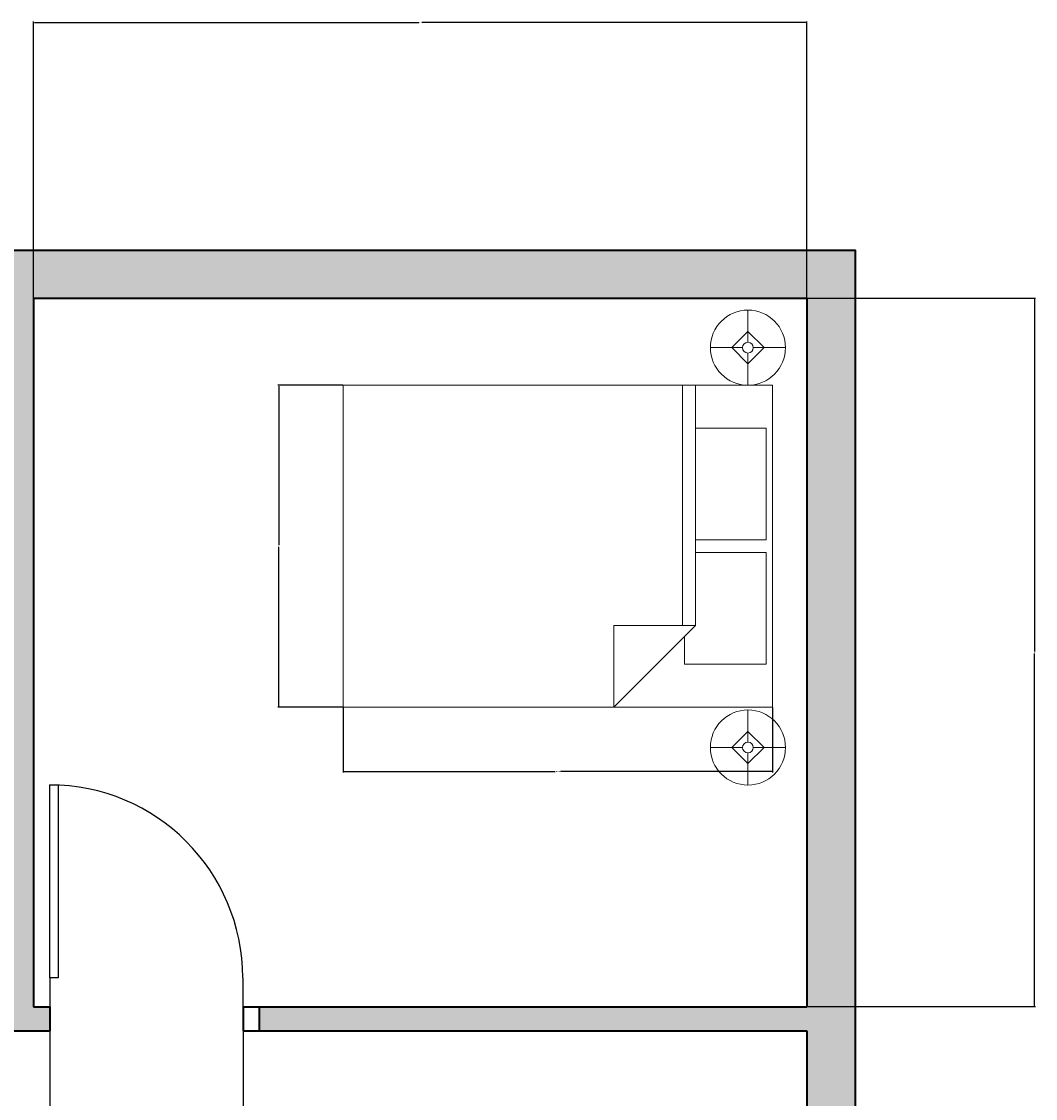
# Model space of a CAD drawing. Units: inches. Extents: x 1563 to 2428, y 777 to 1464.
# Tile 8 of 11: x 1810 to 1999, y 1263 to 1464. Entities that reach past the tile are written whole.
import ezdxf

# ---------------------------------------------------------------- set-up
doc = ezdxf.new("R2010")
doc.units = ezdxf.units.IN
for name, color, linetype, lineweight in [('A-ANNO-DIMS', 2, 'Continuous', 18), ('A-DOOR', 4, 'Continuous', 25), ('A-FURN', 9, 'Continuous', 18), ('A-WALL', 7, 'Continuous', 35), ('A-WALL-PATT', 8, 'Continuous', 13)]:
    doc.layers.add(name, color=color, linetype=linetype, lineweight=lineweight)
doc.styles.get("Standard").update_dxf_attribs({"font": 'arial.ttf'})
doc.dimstyles.get("Standard").update_dxf_attribs({"dimtxt": 0.18, "dimasz": 0.18, "dimexe": 0.18, "dimexo": 0.0625, "dimgap": 0.09, "dimtad": 0, "dimtih": 1, "dimtoh": 1, "dimdec": 4, "dimzin": 0, "dimdsep": 46, "dimtxsty": 'Standard', "dimcen": 0.09, "dimadec": 0, "dimazin": 0, "dimtfac": 1, "dimtdec": 4, "dimtofl": 0, "dimtmove": 0, "dimatfit": 3, "dimfxl": 1, "dimtolj": 1, "dimtzin": 0, "dimarcsym": 0})

# ---------------------------------------------------------------- blocks, each defined once
blk = doc.blocks.new('*U4')
for p, q in [((0, 0), (0, -6)), ((40, 0), (40, -6))]:
    blk.add_line(p, q)
blk.add_lwpolyline([(0, 0), (0, 40), (1.75, 40), (1.75, 0)], close=True)
blk.add_arc((0, 0), 40, 0, 90)
blk = doc.blocks.new('Bed - Queen')
for p, q in [((0, -80.00003), (0, 0)), ((0, 0), (59.99999, 0)), ((59.99999, 0), (59.99999, -80.00003)), ((7.99999, -1.2), (28.79998, -1.2)), ((7.99999, -14.4), (7.99999, -1.2)), ((28.79998, -1.2), (28.79998, -14.4)), ((31.19999, -1.2), (51.99999, -1.2)), ((31.19999, -14.4), (31.19999, -1.2)), ((51.99999, -1.2), (51.99999, -16.4)), ((0, -14.4), (44.8, -14.4)), ((59.99999, -29.6), (44.8, -14.4)), ((44.8, -14.4), (44.8, -29.6)), ((44.8, -16.8), (0, -16.8)), ((51.99999, -16.4), (46.79936, -16.4)), ((44.8, -29.6), (59.99999, -29.6)), ((59.99999, -80.00003), (0, -80.00003))]:
    blk.add_line(p, q)
blk = doc.blocks.new('Lamp - Table')
for p, q in [((0, 7), (0, 1)), ((0, 3), (-3, 0)), ((3, 0), (0, 3)), ((-1, 0), (-7, 0)), ((-3, 0), (0, -3)), ((0, -3), (3, 0)), ((1, 0), (7, 0)), ((0, -1), (0, -7))]:
    blk.add_line(p, q)
for radius in [7, 1]:
    blk.add_circle((0, 0), radius)
blk = doc.blocks.new('*D20')
at = {"layer": 'A-ANNO-DIMS', "color": 0, "lineweight": -2, "transparency": 16777216}
for p, q in [((1869.76, 1336.17), (1869.76, 1324.06)), ((1949.76, 1336.17), (1949.76, 1324.06)), ((1869.94, 1324.24), (1909.25, 1324.24)), ((1949.58, 1324.24), (1910.27, 1324.24))]:
    blk.add_line(p, q, dxfattribs=at)
at = {"layer": 'A-ANNO-DIMS', "color": 0, "transparency": 16777216}
for points in [[(1869.94, 1324.27), (1869.94, 1324.21), (1869.76, 1324.24)], [(1949.58, 1324.27), (1949.58, 1324.21), (1949.76, 1324.24)]]:
    blk.add_solid(points, dxfattribs=at)
at = {"layer": 'Defpoints', "color": 0, "transparency": 16777216}
for p in [(1869.76, 1336.24), (1949.76, 1336.24), (1949.76, 1324.24)]:
    blk.add_point(p, dxfattribs=at)
at = {"layer": 'A-ANNO-DIMS', "color": 0, "transparency": 16777216, "insert": (1909.76, 1324.24), "char_height": 0.18, "attachment_point": 5}
blk.add_mtext('\\A1;BED 80', dxfattribs=at)
blk = doc.blocks.new('*D21')
at = {"layer": 'A-ANNO-DIMS', "color": 0, "lineweight": -2, "transparency": 16777216}
for p, q in [((1869.7, 1396.24), (1857.58, 1396.24)), ((1857.76, 1396.06), (1857.76, 1366.42)), ((1857.76, 1336.42), (1857.76, 1366.05)), ((1869.7, 1336.24), (1857.58, 1336.24))]:
    blk.add_line(p, q, dxfattribs=at)
at = {"layer": 'A-ANNO-DIMS', "color": 0, "transparency": 16777216}
for points in [[(1857.73, 1396.06), (1857.79, 1396.06), (1857.76, 1396.24)], [(1857.73, 1336.42), (1857.79, 1336.42), (1857.76, 1336.24)]]:
    blk.add_solid(points, dxfattribs=at)
at = {"layer": 'Defpoints', "color": 0, "transparency": 16777216}
for p in [(1869.76, 1396.24), (1857.76, 1336.24), (1869.76, 1336.24)]:
    blk.add_point(p, dxfattribs=at)
at = {"layer": 'A-ANNO-DIMS', "color": 0, "transparency": 16777216, "insert": (1857.76, 1366.24), "char_height": 0.18, "attachment_point": 5}
blk.add_mtext('\\A1;60', dxfattribs=at)
blk = doc.blocks.new('*D52')
at = {"layer": 'A-ANNO-DIMS', "color": 0, "lineweight": -2, "transparency": 16777216}
for p, q in [((1812.11, 1412.49), (1812.11, 1464.01)), ((1812.29, 1463.83), (1883.83, 1463.83)), ((1955.93, 1463.83), (1884.39, 1463.83)), ((1956.11, 1412.49), (1956.11, 1464.01))]:
    blk.add_line(p, q, dxfattribs=at)
at = {"layer": 'A-ANNO-DIMS', "color": 0, "transparency": 16777216}
for points in [[(1812.29, 1463.86), (1812.29, 1463.8), (1812.11, 1463.83)], [(1955.93, 1463.86), (1955.93, 1463.8), (1956.11, 1463.83)]]:
    blk.add_solid(points, dxfattribs=at)
at = {"layer": 'Defpoints', "color": 0, "transparency": 16777216}
for p in [(1956.11, 1463.83), (1812.11, 1412.43), (1956.11, 1412.43)]:
    blk.add_point(p, dxfattribs=at)
at = {"layer": 'A-ANNO-DIMS', "color": 0, "transparency": 16777216, "insert": (1884.11, 1463.83), "char_height": 0.18, "attachment_point": 5}
blk.add_mtext('\\A1;144', dxfattribs=at)
blk = doc.blocks.new('*D54')
at = {"layer": 'A-ANNO-DIMS', "color": 0, "lineweight": -2, "transparency": 16777216}
for p, q in [((1956.17, 1412.43), (1998.69, 1412.43)), ((1998.51, 1412.25), (1998.51, 1346.61)), ((1998.51, 1280.61), (1998.51, 1346.25)), ((1956.17, 1280.43), (1998.69, 1280.43))]:
    blk.add_line(p, q, dxfattribs=at)
at = {"layer": 'A-ANNO-DIMS', "color": 0, "transparency": 16777216}
for points in [[(1998.48, 1412.25), (1998.54, 1412.25), (1998.51, 1412.43)], [(1998.48, 1280.61), (1998.54, 1280.61), (1998.51, 1280.43)]]:
    blk.add_solid(points, dxfattribs=at)
at = {"layer": 'Defpoints', "color": 0, "transparency": 16777216}
for p in [(1956.11, 1412.43), (1956.11, 1280.43), (1998.51, 1280.43)]:
    blk.add_point(p, dxfattribs=at)
at = {"layer": 'A-ANNO-DIMS', "color": 0, "transparency": 16777216, "insert": (1998.51, 1346.43), "char_height": 0.18, "attachment_point": 5}
blk.add_mtext('\\A1;132', dxfattribs=at)
blk = doc.blocks.new('*D64')
at = {"layer": 'A-ANNO-DIMS', "color": 0, "lineweight": -2, "transparency": 16777216}
for p, q in [((1815.11, 1275.87), (1815.11, 1233.35)), ((1851.11, 1275.87), (1851.11, 1233.35)), ((1815.29, 1233.53), (1832.89, 1233.53)), ((1850.93, 1233.53), (1833.32, 1233.53))]:
    blk.add_line(p, q, dxfattribs=at)
at = {"layer": 'A-ANNO-DIMS', "color": 0, "transparency": 16777216}
for points in [[(1815.29, 1233.56), (1815.29, 1233.5), (1815.11, 1233.53)], [(1850.93, 1233.56), (1850.93, 1233.5), (1851.11, 1233.53)]]:
    blk.add_solid(points, dxfattribs=at)
at = {"layer": 'Defpoints', "color": 0, "transparency": 16777216}
for p in [(1815.11, 1275.93), (1851.11, 1275.93), (1815.11, 1233.53)]:
    blk.add_point(p, dxfattribs=at)
at = {"layer": 'A-ANNO-DIMS', "color": 0, "transparency": 16777216, "insert": (1833.11, 1233.53), "char_height": 0.18, "attachment_point": 5}
blk.add_mtext('\\A1;36', dxfattribs=at)

msp = doc.modelspace()

# ---------------------------------------------------------------- hatches: boundary and pattern name
at = {"layer": 'A-WALL-PATT'}
h = msp.add_hatch(color=256, dxfattribs=at)
h.dxf.hatch_style = 1
h.paths.add_polyline_path([(1965.105, 1421.428), (1605.105, 1421.428), (1605.105, 821.428), (1965.105, 821.428)])
h.paths.add_polyline_path([(1614.105, 1199.428), (1704.105, 1199.428), (1738.605, 1199.428), (1738.605, 1251.928), (1734.105, 1251.928), (1734.105, 1203.928), (1704.105, 1203.928), (1614.105, 1203.928), (1614.105, 1335.928), (1665.105, 1335.928), (1665.105, 1340.428), (1614.105, 1340.428), (1614.105, 1412.428), (1704.105, 1412.428), (1704.105, 1340.428), (1701.105, 1340.428), (1701.105, 1335.928), (1704.105, 1335.928), (1768.605, 1335.928), (1768.605, 1340.428), (1708.605, 1340.428), (1708.605, 1412.428), (1807.605, 1412.428), (1807.605, 1340.428), (1804.605, 1340.428), (1804.605, 1335.928), (1807.605, 1335.928), (1807.605, 1275.928), (1815.105, 1275.928), (1815.105, 1280.428), (1812.105, 1280.428), (1812.105, 1412.428), (1956.105, 1412.428), (1956.105, 1280.428), (1854.105, 1280.428), (1854.105, 1275.928), (1956.105, 1275.928), (1956.105, 830.428), (1614.105, 830.428)], flags=16)
h.paths.add_polyline_path([(1917.224, 1038.928), (1917.224, 1043.846, -0.4014527), (1951.591, 1079.751), (1951.591, 1079.786), (1953.163, 1079.786), (1953.163, 1043.846), (1953.163, 1038.455), (1953.105, 1034.428), (1953.105, 1038.928), (1953.163, 1043.846), (1951.591, 1043.846), (1951.591, 1079.751, 0.4014527), (1917.224, 1043.846), (1917.224, 1038.455), (1917.224, 1034.428), (1834.605, 1034.428), (1834.605, 906.928), (1858.605, 906.928), (1858.605, 954.928), (1932.105, 954.928), (1932.105, 902.428), (1834.605, 902.428), (1834.605, 1034.428), (1914.224, 1034.428), (1914.224, 1038.928)], flags=0)
edge = h.paths.add_edge_path(flags=0)
edge.add_ellipse((1674.345, 1004.483), major_axis=(1.48, 0), ratio=0.8423039, start_angle=90, end_angle=180, ccw=False)
edge.add_line((1674.345, 1005.73), (1674.921, 1005.73))
edge.add_ellipse((2202.617, 985.642), major_axis=(528.234, 0), ratio=0.8423039, start_angle=176.34957, end_angle=177.82005, ccw=False)
edge.add_ellipse((1739.278, 760.804), major_axis=(-313.308, 0), ratio=0.8423039, start_angle=-77.87403, end_angle=-76.21947, ccw=False)
edge.add_ellipse((1739.278, 767.659), major_axis=(305.303, 0), ratio=0.8423039, start_angle=100.20954, end_angle=102.44463, ccw=False)
edge.add_ellipse((1659.357, 1231.328), major_axis=(250.96, 0), ratio=0.8423039, start_angle=-80.74343, end_angle=-77.44507)
edge.add_line((1705.625, 1023.567), (1711.685, 1026.918))
edge.add_ellipse((1711.754, 1026.21), major_axis=(0.74, 0), ratio=0.8423039, start_angle=52.06687, end_angle=90, ccw=False)
edge.add_line((1712.16, 1026.731), (1717.882, 1023.567))
edge.add_ellipse((1764.151, 1231.328), major_axis=(250.96, 0), ratio=0.8423039, start_angle=257.44507, end_angle=260.74343)
edge.add_ellipse((1684.229, 767.659), major_axis=(305.303, 0), ratio=0.8423039, start_angle=77.55537, end_angle=79.79046, ccw=False)
edge.add_ellipse((1684.229, 760.804), major_axis=(-313.308, 0), ratio=0.8423039, start_angle=256.21947, end_angle=257.87403, ccw=False)
edge.add_ellipse((1220.891, 985.642), major_axis=(-528.234, 0), ratio=0.8423039, start_angle=182.17995, end_angle=183.65043, ccw=False)
edge.add_line((1748.586, 1005.73), (1749.162, 1005.73))
edge.add_ellipse((1749.162, 1004.483), major_axis=(-1.48, 0), ratio=0.8423039, start_angle=180, end_angle=270, ccw=False)
edge.add_line((1750.642, 1004.483), (1750.642, 980.28))
edge.add_ellipse((1749.162, 980.28), major_axis=(1.48, 0), ratio=0.8423039, start_angle=270, end_angle=360, ccw=False)
edge.add_ellipse((-8843.864, 962.352), major_axis=(10593.026, 0), ratio=0.84230387, start_angle=-0.3241203, end_angle=0.0902291, ccw=False)
edge.add_ellipse((-8843.864, 962.352), major_axis=(10593.026, 0), ratio=0.84230387, start_angle=-0.3838668, end_angle=-0.3241203, ccw=False)
edge.add_ellipse((1749.162, 890.136), major_axis=(1.48, 0), ratio=0.8423039, start_angle=0, end_angle=90, ccw=False)
edge.add_line((1750.642, 890.136), (1750.642, 865.933))
edge.add_ellipse((1749.162, 865.933), major_axis=(1.48, 0), ratio=0.8423039, start_angle=270, end_angle=360, ccw=False)
edge.add_line((1749.162, 864.686), (1748.528, 864.686))
edge.add_ellipse((-8843.864, 962.352), major_axis=(10593.026, 0), ratio=0.84230387, start_angle=-0.6186432, end_angle=-0.5282715, ccw=False)
edge.add_ellipse((1747.592, 846.206), major_axis=(-2.22, 0), ratio=0.8423039, start_angle=179.37176, end_angle=248.46476, ccw=False)
edge.add_ellipse((-8844.604, 962.352), major_axis=(-10595.313, 0), ratio=0.842303864, start_angle=179.3534459, end_angle=179.3717628, ccw=False)
edge.add_ellipse((1744.512, 842.854), major_axis=(-5.246, 0), ratio=0.8423039, start_angle=90, end_angle=179.35345, ccw=False)
edge.add_line((1744.512, 838.435), (1678.995, 838.435))
edge.add_ellipse((1678.995, 842.854), major_axis=(5.246, 0), ratio=0.8423039, start_angle=180.64655, end_angle=270, ccw=False)
edge.add_ellipse((12268.111, 962.352), major_axis=(-10595.313, 0), ratio=0.84230387, start_angle=0.6282372, end_angle=0.6465541, ccw=False)
edge.add_ellipse((1675.916, 846.206), major_axis=(-2.22, 0), ratio=0.8423039, start_angle=-68.46476, end_angle=0.62824, ccw=False)
edge.add_ellipse((12267.371, 962.352), major_axis=(-10593.026, 0), ratio=0.84230387, start_angle=0.5282715, end_angle=0.6465541, ccw=False)
edge.add_line((1674.98, 864.686), (1674.345, 864.686))
edge.add_ellipse((1674.345, 865.933), major_axis=(-1.48, 0), ratio=0.8423039, start_angle=0, end_angle=90, ccw=False)
edge.add_line((1672.865, 865.933), (1672.865, 890.136))
edge.add_ellipse((1674.345, 890.136), major_axis=(1.48, 0), ratio=0.8423039, start_angle=90, end_angle=180, ccw=False)
edge.add_ellipse((12267.371, 962.352), major_axis=(-10593.026, 0), ratio=0.84230387, start_angle=0.3241203, end_angle=0.3838668, ccw=False)
edge.add_ellipse((12267.371, 962.352), major_axis=(-10593.026, 0), ratio=0.84230387, start_angle=-0.0902291, end_angle=0.3241203, ccw=False)
edge.add_ellipse((1674.345, 980.28), major_axis=(-1.48, 0), ratio=0.8423039, start_angle=0, end_angle=90, ccw=False)
edge.add_line((1672.865, 980.28), (1672.865, 1004.483))
h.paths.add_polyline_path([(1622.542, 1135.584), (1648.534, 1136.233), (1648.683, 1130.234), (1647.126, 1130.196), (1648.323, 1082.21), (1649.88, 1082.249), (1650.03, 1076.251), (1624.038, 1075.603, -0.266667)], flags=0)
edge = h.paths.add_edge_path(flags=0)
edge.add_line((1694.584, 990.705), (1700.334, 994.711))
edge.add_line((1700.334, 994.711), (1702.248, 994.711))
edge.add_line((1702.248, 994.711), (1702.248, 997.061))
edge.add_ellipse((1758.417, 997.061), major_axis=(56.169, 0), ratio=0.8423039, start_angle=150.56143, end_angle=180, ccw=False)
edge.add_ellipse((1665.091, 997.061), major_axis=(-56.169, 0), ratio=0.8423039, start_angle=180, end_angle=209.43857, ccw=False)
edge.add_line((1721.26, 997.061), (1721.26, 994.711))
edge.add_line((1721.26, 994.711), (1723.174, 994.711))
edge.add_line((1723.174, 994.711), (1728.923, 990.705))
edge.add_line((1728.923, 990.705), (1728.923, 975.895))
edge.add_ellipse((1725.091, 976.043), major_axis=(0.357, 6.34), ratio=0.6038336, start_angle=106.34259, end_angle=270.99799, ccw=False)
edge.add_line((1721.26, 975.15), (1721.26, 997.061))
edge.add_ellipse((1665.091, 997.061), major_axis=(-56.169, 0), ratio=0.8423039, start_angle=180, end_angle=209.43857)
edge.add_ellipse((1758.417, 997.061), major_axis=(56.169, 0), ratio=0.8423039, start_angle=150.56143, end_angle=180)
edge.add_line((1702.248, 997.061), (1702.248, 975.15))
edge.add_ellipse((1698.416, 976.043), major_axis=(-0.357, 6.34), ratio=0.6038336, start_angle=89.00201, end_angle=253.65741, ccw=False)
edge.add_line((1694.584, 975.895), (1694.584, 990.705))
edge = h.paths.add_edge_path(flags=0)
edge.add_line((1675.832, 952.075), (1679.883, 938.848))
edge.add_ellipse((5378.107, 931.045), major_axis=(-3698.236, 0), ratio=0.84230387, start_angle=-0.120897, end_angle=0.364076)
edge.add_line((1679.976, 907.545), (1676.149, 892.52))
edge.add_ellipse((12267.371, 962.352), major_axis=(10591.546, 0), ratio=0.84230387, start_angle=180.3241656, end_angle=180.3777642, ccw=False)
edge.add_ellipse((12267.371, 962.352), major_axis=(10591.546, 0), ratio=0.84230387, start_angle=180.0555943, end_angle=180.3241656, ccw=False)
edge = h.paths.add_edge_path(flags=0)
edge.add_ellipse((1706.366, 891.542), major_axis=(81.773, 0), ratio=0.8423039, start_angle=94.27742, end_angle=111.83495, ccw=False)
edge.add_line((1701.225, 960.283), (1722.283, 960.283))
edge.add_ellipse((1717.141, 891.542), major_axis=(-81.773, 0), ratio=0.8423039, start_angle=248.16505, end_angle=265.72258, ccw=False)
edge.add_line((1743.29, 956.803), (1741.105, 940.427))
edge.add_ellipse((1714.553, 877.238), major_axis=(79.58, 0), ratio=0.8423039, start_angle=67.20809, end_angle=85.12993)
edge.add_line((1720.25, 944.097), (1703.258, 944.097))
edge.add_ellipse((1708.954, 877.238), major_axis=(79.58, 0), ratio=0.8423039, start_angle=94.87007, end_angle=112.79191)
edge.add_line((1682.403, 940.427), (1680.218, 956.803))
h.paths.add_polyline_path([(1664.992, 1093.991), (1664.992, 1123.991), (1724.992, 1123.991), (1724.992, 1093.991)], flags=0)
h.paths.add_polyline_path([(1716.588, 1099.729), (1715.404, 1099.805), (1715.021, 1099.823), (1716.177, 1099.758)], flags=0)
h.paths.add_polyline_path([(1711.325, 1103.757), (1712.167, 1103.706), (1713.009, 1103.642), (1713.84, 1103.566), (1715.041, 1103.439), (1716.532, 1103.244), (1717.793, 1103.048), (1718.876, 1102.854), (1719.676, 1102.699), (1720.157, 1102.605), (1720.632, 1102.513), (1721.109, 1102.424), (1721.595, 1102.339), (1722.088, 1102.264), (1722.585, 1102.205), (1723.082, 1102.17), (1723.575, 1102.164), (1724.321, 1102.211), (1724.533, 1102.268), (1723.842, 1102.16), (1722.864, 1102.172), (1721.894, 1102.287), (1720.935, 1102.454), (1720.157, 1102.605), (1719.676, 1102.699), (1719.18, 1102.795), (1718.66, 1102.892), (1718.109, 1102.991), (1717.517, 1103.091), (1716.876, 1103.191), (1716.179, 1103.29), (1715.435, 1103.387), (1714.652, 1103.48), (1713.84, 1103.566), (1713.009, 1103.642), (1712.167, 1103.706), (1711.325, 1103.757), (1710.492, 1103.791), (1709.676, 1103.806), (1708.873, 1103.805), (1707.707, 1103.78), (1707.292, 1103.757), (1708.499, 1103.805), (1710.086, 1103.807)], flags=0)
h.paths.add_polyline_path([(1713.959, 1106.591), (1714.651, 1106.624), (1715.279, 1106.674), (1715.852, 1106.736), (1716.373, 1106.807), (1716.851, 1106.885), (1717.289, 1106.966), (1717.696, 1107.046), (1718.341, 1107.178), (1719.173, 1107.331), (1720.169, 1107.421), (1721.131, 1107.383), (1722.032, 1107.286), (1722.934, 1107.152), (1723.887, 1106.983), (1724.746, 1106.795), (1724.72, 1106.798), (1724.663, 1106.807), (1724.241, 1106.906), (1724.159, 1106.924), (1723.885, 1106.979), (1723.546, 1107.044), (1723.157, 1107.113), (1722.732, 1107.182), (1722.284, 1107.249), (1721.827, 1107.308), (1721.375, 1107.357), (1720.942, 1107.391), (1720.539, 1107.406), (1720.162, 1107.405), (1719.804, 1107.388), (1719.459, 1107.357), (1719.12, 1107.314), (1718.781, 1107.259), (1718.435, 1107.195), (1718.076, 1107.124), (1717.402, 1106.986), (1716.59, 1106.837), (1715.56, 1106.696), (1714.317, 1106.598)], flags=0)
h.paths.add_polyline_path([(1708.692, 1110.124), (1709.455, 1110.13), (1710.147, 1110.149), (1710.772, 1110.18), (1711.334, 1110.224), (1711.836, 1110.28), (1712.283, 1110.349), (1712.678, 1110.43), (1713.026, 1110.524), (1713.33, 1110.63), (1713.596, 1110.746), (1713.832, 1110.87), (1714.042, 1110.999), (1714.234, 1111.131), (1714.413, 1111.264), (1714.586, 1111.396), (1715.065, 1111.75), (1715.879, 1112.11), (1716.842, 1112.224), (1717.903, 1112.165), (1719.048, 1111.965), (1719.867, 1111.736), (1720.686, 1111.487), (1721.596, 1111.22), (1721.917, 1111.136), (1721.028, 1111.383), (1720.222, 1111.628), (1719.815, 1111.75), (1719.434, 1111.857), (1719.054, 1111.951), (1718.672, 1112.031), (1718.292, 1112.097), (1717.918, 1112.149), (1717.554, 1112.185), (1717.204, 1112.204), (1716.871, 1112.206), (1716.559, 1112.191), (1716.271, 1112.156), (1716.006, 1112.105), (1715.761, 1112.038), (1715.534, 1111.957), (1715.323, 1111.864), (1715.125, 1111.759), (1714.937, 1111.645), (1714.759, 1111.524), (1714.586, 1111.396), (1714.413, 1111.264), (1714.003, 1110.96), (1713.331, 1110.606), (1712.501, 1110.382), (1711.61, 1110.245), (1710.489, 1110.158), (1709.111, 1110.121)], flags=0)
h.paths.add_polyline_path([(1707.127, 1113.075), (1707.639, 1113.025), (1708.092, 1112.991), (1708.49, 1112.975), (1708.836, 1112.977), (1709.135, 1112.996), (1709.392, 1113.032), (1709.612, 1113.084), (1709.798, 1113.15), (1709.957, 1113.23), (1710.092, 1113.324), (1710.208, 1113.431), (1710.304, 1113.554), (1710.379, 1113.698), (1710.434, 1113.866), (1710.467, 1114.062), (1710.477, 1114.289), (1710.463, 1114.553), (1710.426, 1114.857), (1710.364, 1115.202), (1710.282, 1115.58), (1710.184, 1115.98), (1710.076, 1116.391), (1709.961, 1116.801), (1709.844, 1117.201), (1709.731, 1117.579), (1709.626, 1117.924), (1709.532, 1118.228), (1709.454, 1118.493), (1709.392, 1118.723), (1709.351, 1118.924), (1709.293, 1119.435), (1709.831, 1119.942), (1710.705, 1120.121), (1711.507, 1119.898), (1712.224, 1119.567), (1713.189, 1119.016), (1713.529, 1118.804), (1712.958, 1119.148), (1712.468, 1119.428), (1712.046, 1119.649), (1711.683, 1119.817), (1711.366, 1119.937), (1711.084, 1120.016), (1710.826, 1120.057), (1710.582, 1120.067), (1710.354, 1120.049), (1710.142, 1120.006), (1709.951, 1119.941), (1709.781, 1119.857), (1709.635, 1119.757), (1709.516, 1119.645), (1709.426, 1119.524), (1709.366, 1119.395), (1709.335, 1119.255), (1709.331, 1119.1), (1709.351, 1118.924), (1709.392, 1118.723), (1709.454, 1118.493), (1709.52, 1118.268), (1709.799, 1117.356), (1710.028, 1116.57), (1710.245, 1115.749), (1710.45, 1114.804), (1710.477, 1114.289), (1710.448, 1113.654), (1709.908, 1113.153), (1709.165, 1112.979), (1708.318, 1112.974), (1707.448, 1113.039)], flags=0)
h.paths.add_polyline_path([(1700.892, 1119.857), (1701.604, 1119.819), (1702.196, 1119.805), (1702.683, 1119.813), (1703.076, 1119.841), (1703.387, 1119.887), (1703.63, 1119.951), (1703.816, 1120.03), (1703.959, 1120.124), (1704.069, 1120.23), (1704.15, 1120.346), (1704.204, 1120.47), (1704.234, 1120.599), (1704.242, 1120.731), (1704.231, 1120.864), (1704.202, 1120.996), (1704.159, 1121.124), (1704.103, 1121.246), (1704.039, 1121.362), (1703.97, 1121.474), (1703.901, 1121.582), (1703.834, 1121.687), (1703.775, 1121.79), (1703.564, 1122.226), (1704.048, 1122.698), (1704.756, 1122.769), (1705.49, 1122.723), (1706.24, 1122.641), (1706.547, 1122.601), (1706.092, 1122.657), (1705.695, 1122.701), (1705.348, 1122.732), (1705.049, 1122.751), (1704.792, 1122.757), (1704.573, 1122.751), (1704.386, 1122.732), (1704.227, 1122.701), (1704.092, 1122.657), (1703.977, 1122.601), (1703.88, 1122.534), (1703.802, 1122.458), (1703.742, 1122.374), (1703.702, 1122.284), (1703.68, 1122.188), (1703.677, 1122.09), (1703.692, 1121.991), (1703.726, 1121.89), (1703.769, 1121.802), (1704.039, 1121.362), (1704.301, 1120.887), (1704.133, 1120.165), (1703.43, 1119.866), (1702.481, 1119.798), (1701.306, 1119.827)], flags=0)
edge = h.paths.add_edge_path(flags=0)
edge.add_ellipse((1711.754, 1009.752), major_axis=(-147.018, 0), ratio=0.8423039, start_angle=76.40187, end_angle=103.59813)
edge.add_line((1741.105, 888.411), (1741.105, 869.587))
edge.add_ellipse((1711.754, 990.928), major_axis=(-147.018, 0), ratio=0.8423039, start_angle=76.40187, end_angle=103.59813, ccw=False)
edge.add_line((1682.403, 869.587), (1682.403, 888.411))
edge = h.paths.add_edge_path(flags=0)
edge.add_ellipse((-8843.864, 962.352), major_axis=(-10591.546, 0), ratio=0.84230387, start_angle=179.6758344, end_angle=179.9444057, ccw=False)
edge.add_ellipse((-8843.864, 962.352), major_axis=(-10591.546, 0), ratio=0.84230387, start_angle=179.6222358, end_angle=179.6758344, ccw=False)
edge.add_line((1747.358, 892.52), (1743.531, 907.545))
edge.add_ellipse((-1954.6, 931.045), major_axis=(3698.236, 0), ratio=0.84230387, start_angle=-0.364076, end_angle=0.120897)
edge.add_line((1743.625, 938.848), (1747.676, 952.075))
h.paths.add_polyline_path([(1637.931, 1162.087), (1637.931, 1188.087, -0.1904762), (1721.931, 1188.087), (1721.931, 1162.087), (1715.931, 1162.087), (1715.931, 1163.644), (1643.931, 1163.644), (1643.931, 1162.087)], flags=0)
h.paths.add_polyline_path([(1667.931, 1189.491, -0.0496282), (1691.931, 1189.491), (1691.931, 1182.705), (1667.931, 1182.705)], flags=0)
edge = h.paths.add_edge_path(flags=0)
edge.add_ellipse((1685.362, 859.825), major_axis=(-2.96, 0), ratio=0.8423039, start_angle=-90, end_angle=0, ccw=False)
edge.add_line((1685.362, 862.318), (1738.145, 862.318))
edge.add_ellipse((1738.145, 859.825), major_axis=(2.96, 0), ratio=0.8423039, start_angle=0, end_angle=90, ccw=False)
edge.add_line((1741.105, 859.825), (1741.105, 840.361))
edge.add_line((1741.105, 840.361), (1682.403, 840.361))
edge.add_line((1682.403, 840.361), (1682.403, 859.825))
h.paths.add_polyline_path([(1777.486, 1164.853), (1777.486, 1180.853), (1778.486, 1181.01), (1778.486, 1164.697)], flags=0)
h.paths.add_polyline_path([(1786.986, 1154.853), (1786.986, 1163.369), (1778.986, 1164.619), (1778.986, 1181.088), (1786.986, 1182.338), (1786.986, 1190.853), (1799.502, 1190.853), (1800.752, 1198.853), (1817.221, 1198.853), (1818.471, 1190.853), (1827.502, 1190.853), (1828.752, 1198.853), (1845.221, 1198.853), (1846.471, 1190.853), (1858.986, 1190.853), (1858.986, 1182.338), (1866.986, 1181.088), (1866.986, 1164.619), (1858.986, 1163.369), (1858.986, 1154.853), (1846.471, 1154.853), (1845.221, 1146.853), (1828.752, 1146.853), (1827.502, 1154.853), (1818.471, 1154.853), (1817.221, 1146.853), (1800.752, 1146.853), (1799.502, 1154.853)], flags=0)
h.paths.add_polyline_path([(1800.986, 1145.353), (1800.83, 1146.353), (1817.143, 1146.353), (1816.986, 1145.353)], flags=0)
h.paths.add_polyline_path([(1851.408, 1167.858), (1852.086, 1167.738), (1852.744, 1167.621), (1853.388, 1167.506), (1854.028, 1167.395), (1854.67, 1167.289), (1855.313, 1167.195), (1855.952, 1167.122), (1856.585, 1167.077), (1857.209, 1167.07), (1858.147, 1167.128), (1858.413, 1167.2), (1857.547, 1167.066), (1856.312, 1167.08), (1855.07, 1167.223), (1854.028, 1167.395), (1853.388, 1167.506), (1852.744, 1167.621), (1852.086, 1167.738), (1851.408, 1167.858), (1850.288, 1168.052), (1849.956, 1168.104), (1850.701, 1167.98)], flags=0)
h.paths.add_polyline_path([(1845.435, 1172.646), (1846.222, 1172.707), (1846.941, 1172.785), (1847.601, 1172.874), (1848.21, 1172.971), (1848.777, 1173.072), (1849.311, 1173.173), (1850.14, 1173.331), (1851.063, 1173.483), (1852.014, 1173.591), (1853.012, 1173.633), (1854.075, 1173.594), (1855.251, 1173.473), (1856.4, 1173.306), (1857.391, 1173.132), (1857.945, 1173.02), (1858.196, 1172.965), (1858.595, 1172.871), (1858.575, 1172.874), (1858.49, 1172.894), (1858.371, 1172.924), (1858.196, 1172.965), (1857.945, 1173.02), (1857.602, 1173.089), (1857.177, 1173.17), (1856.687, 1173.256), (1856.148, 1173.343), (1855.575, 1173.426), (1854.986, 1173.5), (1854.395, 1173.561), (1853.82, 1173.603), (1853.272, 1173.623), (1852.749, 1173.622), (1852.247, 1173.6), (1851.757, 1173.562), (1851.276, 1173.507), (1850.796, 1173.439), (1850.313, 1173.359), (1849.82, 1173.27), (1849.311, 1173.173), (1848.421, 1173.005), (1847.25, 1172.818), (1845.826, 1172.665)], flags=0)
h.paths.add_polyline_path([(1840.587, 1177.09), (1841.289, 1177.145), (1841.916, 1177.215), (1842.475, 1177.301), (1842.969, 1177.403), (1843.403, 1177.52), (1843.783, 1177.652), (1844.117, 1177.797), (1844.411, 1177.952), (1844.674, 1178.114), (1844.914, 1178.279), (1845.138, 1178.446), (1845.644, 1178.831), (1846.285, 1179.221), (1847.125, 1179.521), (1847.998, 1179.624), (1848.834, 1179.619), (1849.768, 1179.529), (1850.775, 1179.363), (1851.78, 1179.14), (1852.111, 1179.053), (1851.57, 1179.187), (1851.043, 1179.304), (1850.527, 1179.404), (1850.024, 1179.487), (1849.539, 1179.551), (1849.072, 1179.596), (1848.628, 1179.62), (1848.21, 1179.623), (1847.82, 1179.603), (1847.46, 1179.561), (1847.128, 1179.497), (1846.822, 1179.413), (1846.539, 1179.312), (1846.274, 1179.195), (1846.027, 1179.064), (1845.793, 1178.922), (1845.57, 1178.77), (1845.354, 1178.61), (1844.817, 1178.201), (1844.106, 1177.764), (1843.208, 1177.452), (1842.225, 1177.25), (1840.973, 1177.11)], flags=0)
h.paths.add_polyline_path([(1836.67, 1180.646), (1837.236, 1180.603), (1837.734, 1180.584), (1838.166, 1180.586), (1838.54, 1180.611), (1838.861, 1180.655), (1839.136, 1180.72), (1839.369, 1180.803), (1839.568, 1180.903), (1839.736, 1181.02), (1839.881, 1181.152), (1840.001, 1181.299), (1840.095, 1181.456), (1840.164, 1181.624), (1840.204, 1181.8), (1840.217, 1181.981), (1840.2, 1182.166), (1840.153, 1182.353), (1840.076, 1182.541), (1839.973, 1182.728), (1839.851, 1182.916), (1839.716, 1183.103), (1839.572, 1183.291), (1839.427, 1183.478), (1839.033, 1184), (1838.862, 1184.411), (1838.695, 1184.99), (1839.2, 1185.669), (1840.06, 1185.961), (1840.793, 1185.931), (1841.454, 1185.77), (1842.179, 1185.536), (1842.706, 1185.363), (1843.713, 1185.044), (1844.033, 1184.956), (1843.102, 1185.234), (1842.179, 1185.536), (1841.725, 1185.682), (1841.328, 1185.801), (1840.976, 1185.886), (1840.653, 1185.937), (1840.349, 1185.949), (1840.063, 1185.926), (1839.799, 1185.872), (1839.559, 1185.791), (1839.347, 1185.686), (1839.165, 1185.562), (1839.016, 1185.422), (1838.903, 1185.27), (1838.828, 1185.11), (1838.79, 1184.943), (1838.784, 1184.77), (1838.809, 1184.593), (1838.862, 1184.411), (1838.938, 1184.227), (1839.036, 1184.041), (1839.153, 1183.853), (1839.285, 1183.666), (1839.427, 1183.478), (1839.572, 1183.291), (1839.716, 1183.103), (1839.851, 1182.916), (1840.178, 1182.415), (1840.251, 1181.604), (1839.686, 1180.915), (1838.893, 1180.633), (1837.976, 1180.574), (1837.01, 1180.612)], flags=0)
h.paths.add_polyline_path([(1829.867, 1185.622), (1830.475, 1185.631), (1830.966, 1185.666), (1831.355, 1185.724), (1831.658, 1185.804), (1831.891, 1185.903), (1832.07, 1186.02), (1832.207, 1186.152), (1832.308, 1186.297), (1832.376, 1186.452), (1832.414, 1186.614), (1832.424, 1186.779), (1832.41, 1186.946), (1832.374, 1187.11), (1832.32, 1187.27), (1832.25, 1187.422), (1832.17, 1187.568), (1832.084, 1187.708), (1831.997, 1187.843), (1831.914, 1187.974), (1831.839, 1188.102), (1831.614, 1188.57), (1832.036, 1189.169), (1832.801, 1189.319), (1833.589, 1189.3), (1834.44, 1189.223), (1834.736, 1189.187), (1834.239, 1189.241), (1833.807, 1189.28), (1833.433, 1189.304), (1833.111, 1189.312), (1832.837, 1189.304), (1832.604, 1189.28), (1832.405, 1189.241), (1832.236, 1189.187), (1832.092, 1189.117), (1831.971, 1189.033), (1831.873, 1188.938), (1831.799, 1188.832), (1831.748, 1188.719), (1831.721, 1188.601), (1831.717, 1188.478), (1831.736, 1188.353), (1831.779, 1188.228), (1831.839, 1188.102), (1831.914, 1187.974), (1831.997, 1187.843), (1832.084, 1187.708), (1832.387, 1187.216), (1832.456, 1186.393), (1831.916, 1185.871), (1831.195, 1185.682), (1830.221, 1185.613)], flags=0)
h.paths.add_polyline_path([(1828.986, 1145.353), (1828.83, 1146.353), (1845.143, 1146.353), (1844.986, 1145.353)], flags=0)
h.paths.add_polyline_path([(1800.986, 1200.353), (1816.986, 1200.353), (1817.143, 1199.353), (1800.83, 1199.353)], flags=0)
h.paths.add_polyline_path([(1828.986, 1200.353), (1844.986, 1200.353), (1845.143, 1199.353), (1828.83, 1199.353)], flags=0)
h.paths.add_polyline_path([(1867.486, 1181.01), (1868.486, 1180.853), (1868.486, 1164.853), (1867.486, 1164.697)], flags=0)
h.paths.add_polyline_path([(1901.055, 1112.089), (1901.055, 1241.889), (1954.299, 1241.889), (1954.299, 1112.089)], flags=0)
h.paths.add_polyline_path([(1908.544, 1229.408), (1931.009, 1229.408), (1937.23, 1216.927), (1931.009, 1216.927), (1931.009, 1129.562), (1908.544, 1129.562)], flags=0)
h.paths.add_polyline_path([(1699.472, 1381.538), (1701.045, 1381.538), (1701.045, 1345.599), (1699.472, 1345.599)], flags=0)
h.paths.add_polyline_path([(1851.045, 1285.819), (1851.045, 1280.428), (1851.105, 1275.928), (1851.105, 1280.428)], flags=0)
h.paths.add_polyline_path([(1815.105, 1285.819), (1815.105, 1321.758), (1816.678, 1321.758), (1816.678, 1285.819)], flags=0)
h.paths.add_polyline_path([(1745.154, 1343.707, -0.1044693), (1742.568, 1347.148, -0.1176343), (1741.799, 1350.905, -0.1176343), (1742.808, 1354.603, -0.1044693), (1745.61, 1357.871, -0.0900158), (1749.544, 1359.891, -0.0819199), (1754.355, 1360.526, -0.0819199), (1759.115, 1359.583, -0.0900158), (1762.911, 1357.314, -0.1044693), (1765.497, 1353.872, -0.1176343), (1766.266, 1350.116, -0.1176343), (1765.257, 1346.417, -0.1044693), (1762.455, 1343.149, -0.0900158), (1758.521, 1341.13, -0.0819199), (1753.71, 1340.495, -0.0819199), (1748.95, 1341.438, -0.0900158)], flags=0)
h.paths.add_polyline_path([(1745.961, 1344.152, -0.1046782), (1743.517, 1347.257, -0.1186217), (1742.746, 1350.669, -0.1186217), (1743.612, 1354.059, -0.1046782), (1746.143, 1357.094, -0.0895621), (1749.732, 1359.002, -0.0811847), (1754.161, 1359.662, -0.0811847), (1758.57, 1358.877, -0.0895621), (1762.104, 1356.869, -0.1046782), (1764.548, 1353.764, -0.1186217), (1765.319, 1350.351, -0.1186217), (1764.453, 1346.962, -0.1046782), (1761.922, 1343.927, -0.0895621), (1758.333, 1342.019, -0.0811847), (1753.904, 1341.359, -0.0811847), (1749.495, 1342.143, -0.0895621)], flags=0)
h.paths.add_polyline_path([(1748.738, 1346.3, -0.1046075), (1747.125, 1348.343, -0.1182826), (1746.612, 1350.593, -0.1182826), (1747.176, 1352.832, -0.1046075), (1748.833, 1354.838, -0.089718), (1751.19, 1356.103, -0.0814361), (1754.1, 1356.547, -0.0814361), (1756.999, 1356.038, -0.089718), (1759.327, 1354.72, -0.1046075), (1760.94, 1352.678, -0.1182826), (1761.453, 1350.427, -0.1182826), (1760.889, 1348.189, -0.1046075), (1759.232, 1346.183, -0.089718), (1756.875, 1344.917, -0.0814361), (1753.965, 1344.474, -0.0814361), (1751.066, 1344.982, -0.089718)], flags=0)
h.paths.add_polyline_path([(1802.972, 1381.538), (1804.545, 1381.538), (1804.545, 1345.599), (1802.972, 1345.599)], flags=0)
h.paths.add_polyline_path([(1752.533, 1350.51, -1), (1755.533, 1350.51, -1)], flags=0)
h.paths.add_polyline_path([(1753.033, 1350.51, -1), (1755.033, 1350.51, -1)], flags=0)
h.paths.add_polyline_path([(1869.759, 1336.236), (1869.759, 1396.236), (1949.759, 1396.236), (1949.759, 1336.236)], flags=0)
h.paths.add_polyline_path([(1920.159, 1336.236), (1920.159, 1351.436), (1935.359, 1351.436), (1935.359, 1388.236), (1948.559, 1388.236), (1948.559, 1367.436), (1935.359, 1367.436), (1935.359, 1365.036), (1948.559, 1365.036), (1948.559, 1344.236), (1933.359, 1344.236), (1933.359, 1349.436)], flags=0)
h.paths.add_polyline_path([(1938.156, 1328.719, -1), (1952.156, 1328.719, -1)], flags=0)
h.paths.add_polyline_path([(1942.156, 1328.719), (1945.156, 1331.719), (1948.156, 1328.719), (1945.156, 1325.719)], flags=0)
h.paths.add_polyline_path([(1944.156, 1328.719, -1), (1946.156, 1328.719, -1)], flags=0)
h.paths.add_polyline_path([(1914.224, 1038.928), (1614.105, 1038.928), (1614.105, 1034.428), (1830.105, 1034.428), (1830.105, 830.428), (1834.605, 830.428), (1834.605, 1034.428), (1914.224, 1034.428)], flags=0)
h.paths.add_polyline_path([(1956.105, 902.428), (1834.605, 902.428), (1834.605, 830.428), (1956.105, 830.428)], flags=0)

# ---------------------------------------------------------------- linework, layer by layer
at = {"layer": 'A-WALL'}
for p, q in [((1812.105, 1412.428), (1812.105, 1280.428)), ((1812.105, 1412.428), (1956.105, 1412.428)), ((1956.105, 1412.428), (1956.105, 1280.428)), ((1812.105, 1280.428), (1815.105, 1280.428)), ((1815.105, 1280.428), (1815.105, 1275.928)), ((1851.105, 1280.428), (1851.105, 1275.928)), ((1851.105, 1280.428), (1956.105, 1280.428)), ((1854.105, 1280.428), (1854.105, 1275.928)), ((1807.605, 1275.928), (1815.105, 1275.928)), ((1851.105, 1275.928), (1956.105, 1275.928)), ((1956.105, 1275.928), (1956.105, 830.428))]:
    msp.add_line(p, q, dxfattribs=at)
msp.add_lwpolyline([(1605.105, 1421.428), (1965.105, 1421.428), (1965.105, 821.428), (1605.105, 821.428)], close=True, dxfattribs=at)

# ---------------------------------------------------------------- block references
at = {"layer": 'A-DOOR', "xscale": 0.8984802532018953, "yscale": 0.8984802532018953, "zscale": 0.8984802532018953}
msp.add_blockref('*U4', (1815.105, 1285.819), dxfattribs=at)
at = {"layer": 'A-FURN'}
for p in [(1945.156, 1403.236), (1945.156, 1328.719)]:
    msp.add_blockref('Lamp - Table', p, dxfattribs=at)
at = {"layer": 'A-FURN', "rotation": 270}
msp.add_blockref('Bed - Queen', (1949.759, 1396.236), dxfattribs=at)

# ---------------------------------------------------------------- dimensions: what is measured, and where the dimension line sits
at = {"layer": 'A-ANNO-DIMS'}
dim = msp.add_linear_dim(base=(1956.105, 1463.828), p1=(1812.105, 1412.428), p2=(1956.105, 1412.428), dimstyle='Standard', override={"dimdec": 0, "dimlfac": 1, "dimrnd": 0, "dimzin": 0, "dimdsep": 46, "dimlunit": 2}, dxfattribs=at)
dim.commit()
dim.dimension.update_dxf_attribs({"geometry": '*D52', "text_midpoint": (1884.105, 1463.828)})
for base, p1, p2, angle, picture, middle in [((1998.505, 1280.428), (1956.105, 1412.428), (1956.105, 1280.428), 270, '*D54', (1998.505, 1346.428)), ((1857.759, 1336.236), (1869.759, 1396.236), (1869.759, 1336.236), 270, '*D21', (1857.759, 1366.236)), ((1815.105, 1233.528), (1851.105, 1275.928), (1815.105, 1275.928), 180, '*D64', (1833.105, 1233.528))]:
    dim = msp.add_linear_dim(base=base, p1=p1, p2=p2, angle=angle, dimstyle='Standard', override={"dimdec": 0, "dimlfac": 1, "dimrnd": 0, "dimzin": 0, "dimdsep": 46, "dimlunit": 2}, dxfattribs=at)
    dim.commit()
    dim.dimension.update_dxf_attribs({"geometry": picture, "text_midpoint": middle})
dim = msp.add_linear_dim(base=(1949.759, 1324.236), p1=(1869.759, 1336.236), p2=(1949.759, 1336.236), text='BED <>', dimstyle='Standard', override={"dimdec": 0, "dimlfac": 1, "dimrnd": 0, "dimzin": 0, "dimdsep": 46, "dimlunit": 2}, dxfattribs=at)
dim.commit()
dim.dimension.update_dxf_attribs({"geometry": '*D20', "text_midpoint": (1909.759, 1324.236)})

doc.saveas('drawing.dxf')
